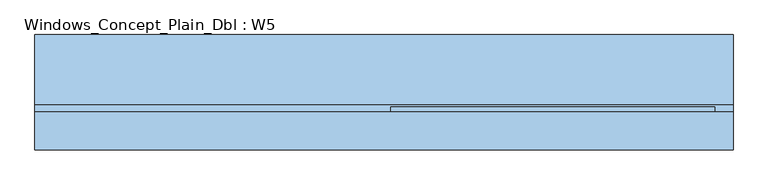
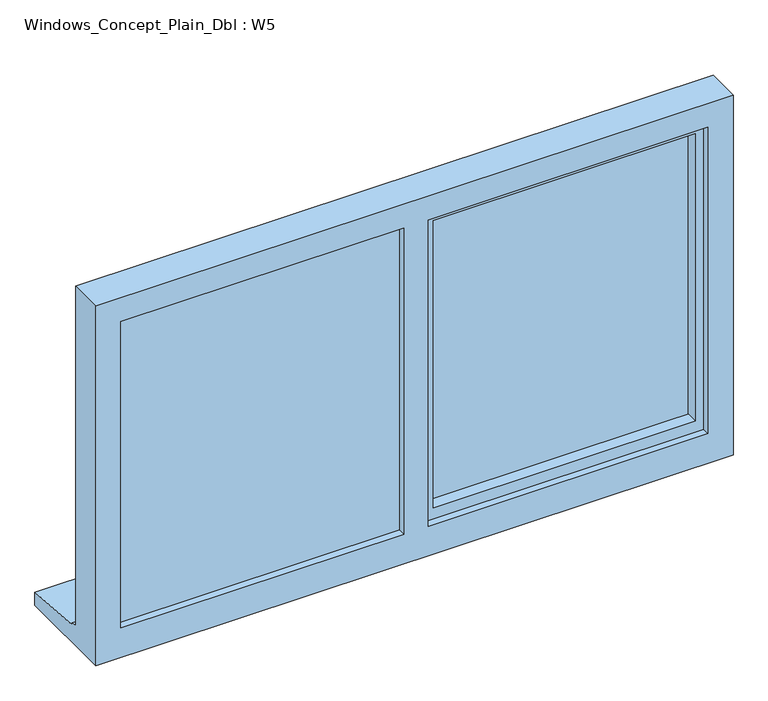
"""IFC4 building model written with IfcOpenShell, lengths in millimetres: window geometry, Windows_Concept_Plain_Dbl : W5."""

from ifc_helpers import new_model, si_unit, frame, origin, place, context, project, spatial, polyline, outline, extrude, faceted_brep, source, transform, mapped, element, save


def windows_concept_plain_dbl_w5_831b8d9f(model_context):
    return source(origin(), model_context, "Body", "SolidModel", [
        faceted_brep([(-270.0, -37.9634322, 2070.0), (-270.0, 38.5835732, 2070.0), (-270.0, 38.5835732, 1263.0), (-270.0, -37.9634322, 1263.0), (-230.0, -8.9634322, 2030.0), (-230.0, -37.9634322, 2030.0), (-230.0, -37.9634322, 1303.0), (-230.0, -8.9634322, 1303.0), (-240.0, 15.0365678, 2040.0), (-240.0, -8.9634322, 2040.0), (-240.0, -8.9634322, 1293.0), (-240.0, 15.0365678, 1293.0), (-230.0, 38.5835732, 2030.0), (-230.0, 15.0365678, 2030.0), (-230.0, 15.0365678, 1303.0), (-230.0, 38.5835732, 1303.0), (437.0, 38.5835732, 1263.0), (437.0, -37.9634322, 1263.0), (397.0, -37.9634322, 1303.0), (397.0, -8.9634322, 1303.0), (407.0, -8.9634322, 1293.0), (407.0, 15.0365678, 1293.0), (397.0, 15.0365678, 1303.0), (397.0, 38.5835732, 1303.0), (437.0, 38.5835732, 2070.0), (437.0, -37.9634322, 2070.0), (397.0, -37.9634322, 2030.0), (397.0, -8.9634322, 2030.0), (407.0, -8.9634322, 2040.0), (407.0, 15.0365678, 2040.0), (397.0, 15.0365678, 2030.0), (397.0, 38.5835732, 2030.0)], [[[0, 1, 2, 3]], [[4, 5, 6, 7]], [[8, 9, 10, 11]], [[12, 13, 14, 15]], [[3, 2, 16, 17]], [[7, 6, 18, 19]], [[11, 10, 20, 21]], [[15, 14, 22, 23]], [[17, 16, 24, 25]], [[19, 18, 26, 27]], [[21, 20, 28, 29]], [[23, 22, 30, 31]], [[1, 24, 16, 2], [15, 23, 31, 12]], [[25, 24, 1, 0]], [[3, 17, 25, 0], [5, 26, 18, 6]], [[27, 26, 5, 4]], [[9, 28, 20, 10], [7, 19, 27, 4]], [[29, 28, 9, 8]], [[11, 21, 29, 8], [13, 30, 22, 14]], [[31, 30, 13, 12]]]),
        extrude(outline(polyline([(2050.0, -310.0), (2070.0, -310.0), (2070.0, -1007.0), (1263.0, -1007.0), (1263.0, -310.0), (1283.0, -310.0), (1283.0, -987.0), (2050.0, -987.0), (2050.0, -310.0)])), frame((0.0, -13.9634322, 0.0), z_axis=(0.0, 1.0, 0.0), x_axis=(0.0, 0.0, 1.0)), (0.0, 0.0, 1.0), 41.0),
        faceted_brep([(477.0, -55.9634322, 2110.0), (-1047.0, -55.9634322, 2110.0), (-1047.0, -55.9634322, 1200.0), (477.0, -55.9634322, 1200.0), (417.0, -55.9634322, 2050.0), (417.0, -55.9634322, 1275.0), (-252.0, -55.9634322, 1275.0), (-252.0, -55.9634322, 2050.0), (-310.0, -55.9634322, 2050.0), (-310.0, -55.9634322, 1275.0), (-987.0, -55.9634322, 1275.0), (-987.0, -55.9634322, 2050.0), (-1047.0, 27.0365678, 2110.0), (-1047.0, 27.0365678, 1251.0), (-1047.0, 42.0365678, 1249.68767), (-1047.0, 42.0365678, 1244.7449676), (-1047.0, 195.9565678, 1233.8088847), (-1047.0, 195.9565678, 1200.0), (477.0, 27.0365678, 2110.0), (477.0, 27.0365678, 1251.0), (-1007.0, 27.0365678, 2070.0), (-1007.0, 27.0365678, 1263.0), (-310.0, 27.0365678, 1263.0), (-310.0, 27.0365678, 2070.0), (-270.0, 27.0365678, 2070.0), (-270.0, 27.0365678, 1263.0), (437.0, 27.0365678, 1263.0), (437.0, 27.0365678, 2070.0), (-1007.0, -37.9634322, 2070.0), (-1007.0, -37.9634322, 1263.0), (-300.0, -37.9634322, 2070.0), (-300.0, -37.9634322, 1263.0), (-310.0, -37.9634322, 2050.0), (-987.0, -37.9634322, 2050.0), (-987.0, -37.9634322, 1275.0), (-310.0, -37.9634322, 1275.0), (-270.0, -37.9634322, 2070.0), (437.0, -37.9634322, 2070.0), (437.0, -37.9634322, 1263.0), (-270.0, -37.9634322, 1263.0), (417.0, -37.9634322, 2050.0), (-252.0, -37.9634322, 2050.0), (-252.0, -37.9634322, 1275.0), (417.0, -37.9634322, 1275.0), (-310.0, -13.9634322, 2070.0), (-300.0, -13.9634322, 2070.0), (477.0, 195.9565678, 1200.0), (477.0, 195.9565678, 1233.8088847), (477.0, 42.0365678, 1244.7449676), (477.0, 42.0365678, 1249.68767), (-300.0, -13.9634322, 1263.0), (-310.0, -13.9634322, 1263.0)], [[[0, 1, 2, 3], [4, 5, 6, 7], [8, 9, 10, 11]], [[2, 1, 12, 13, 14, 15, 16, 17]], [[13, 12, 18, 19], [20, 21, 22, 23], [24, 25, 26, 27]], [[21, 20, 28, 29]], [[28, 30, 31, 29], [32, 33, 34, 35]], [[36, 37, 38, 39], [40, 41, 42, 43]], [[33, 11, 10, 34]], [[1, 0, 18, 12]], [[28, 20, 23, 44, 45, 30]], [[27, 37, 36, 24]], [[11, 33, 32, 8]], [[40, 4, 7, 41]], [[19, 18, 0, 3, 46, 47, 48, 49]], [[27, 26, 38, 37]], [[4, 40, 43, 5]], [[45, 50, 31, 30]], [[50, 45, 44, 51]], [[51, 44, 23, 22]], [[25, 24, 36, 39]], [[41, 7, 6, 42]], [[8, 32, 35, 9]], [[46, 3, 2, 17]], [[47, 46, 17, 16]], [[48, 47, 16, 15]], [[49, 48, 15, 14]], [[19, 49, 14, 13]], [[22, 21, 29, 31, 50, 51]], [[26, 25, 39, 38]], [[6, 5, 43, 42]], [[35, 34, 10, 9]]]),
        extrude(outline(polyline([(-1007.0, -13.9634322), (-300.0, -13.9634322), (-300.0, -37.9634322), (-1007.0, -37.9634322), (-1007.0, -13.9634322)])), frame((0.0, 0.0, 1263.0), z_axis=(0.0, 0.0, 1.0), x_axis=(1.0, 0.0, 0.0)), (0.0, 0.0, 1.0), 807.0),
        extrude(outline(polyline([(407.0, -8.9634322), (-240.0, -8.9634322), (-240.0, 15.0365678), (407.0, 15.0365678), (407.0, -8.9634322)])), frame((0.0, 0.0, 1293.0), z_axis=(0.0, 0.0, 1.0), x_axis=(1.0, 0.0, 0.0)), (0.0, 0.0, 1.0), 747.0),
    ])


if __name__ == "__main__":
    model = new_model("IFC4")
    model_context = context("Model", 3, world=origin())
    ifc_project = project(units=[si_unit("LENGTHUNIT", "METRE", prefix="MILLI")], contexts=[model_context])
    site = spatial("IfcSite", under=ifc_project)
    building = spatial("IfcBuilding", under=site)
    placement = place(None, origin())
    windows_concept_plain_dbl_w5_shape = windows_concept_plain_dbl_w5_831b8d9f(model_context)
    element("IfcWindow", 1, ObjectType="Windows_Concept_Plain_Dbl : W5", at=placement, inside=building, context=model_context, shape_type="MappedRepresentation", body=[
        mapped(windows_concept_plain_dbl_w5_shape, transform((0.0, 0.0, 0.0), x_axis=(1.0, 0.0, 0.0), y_axis=(0.0, 1.0, 0.0), z_axis=(0.0, 0.0, 1.0))),
    ])
    save(model, "model.ifc")

# Revit data of these elements
# Type "Windows_Concept_Plain_Dbl : W5"
#   Type Mark = "60"
#   Operation = "DoublePanelVertical"
#   Construction Type Id = "GSP4R"
#   Manufacturer = "Revit"
#   Keynote = "L10"
#   Analytic Construction = "1/8 in Pilkington single glazing"
#   Visual Light Transmittance = 0.9
#   Solar Heat Gain Coefficient = 0.78
#   Rough Width = 1524 mm
#   Rough Height = 910 mm
#   Height = 910 mm
#   Width = 1524 mm
#   Heat Transfer Coefficient (U) = 3.6886 W/(m²·K)
#   FrameOffset - External = 50 mm
#   Default Head Height = 2110 mm
#   Vis - Cavity Closers = yes
#   Define Thermal Properties by = 1
#   Material Trim = Window Frame
#   Material Glass = Glass
#   Material Frame = Window Frame
#   Wall Closure = (empty or 0)
# Element 1 (IfcWindow, "Windows_Concept_Plain_Dbl : W5")
#   Materials on its faces: "Window Frame", "Glass"
# Materials
#   "Window Frame": colour RGB 249 249 249, transparency 0, Keynote = "L10", Cost = 0
#   "Glass": class "Glass", colour RGB 0 128 192, transparency 0.9, Description = "Soda Lime Glass", Cost = 0
